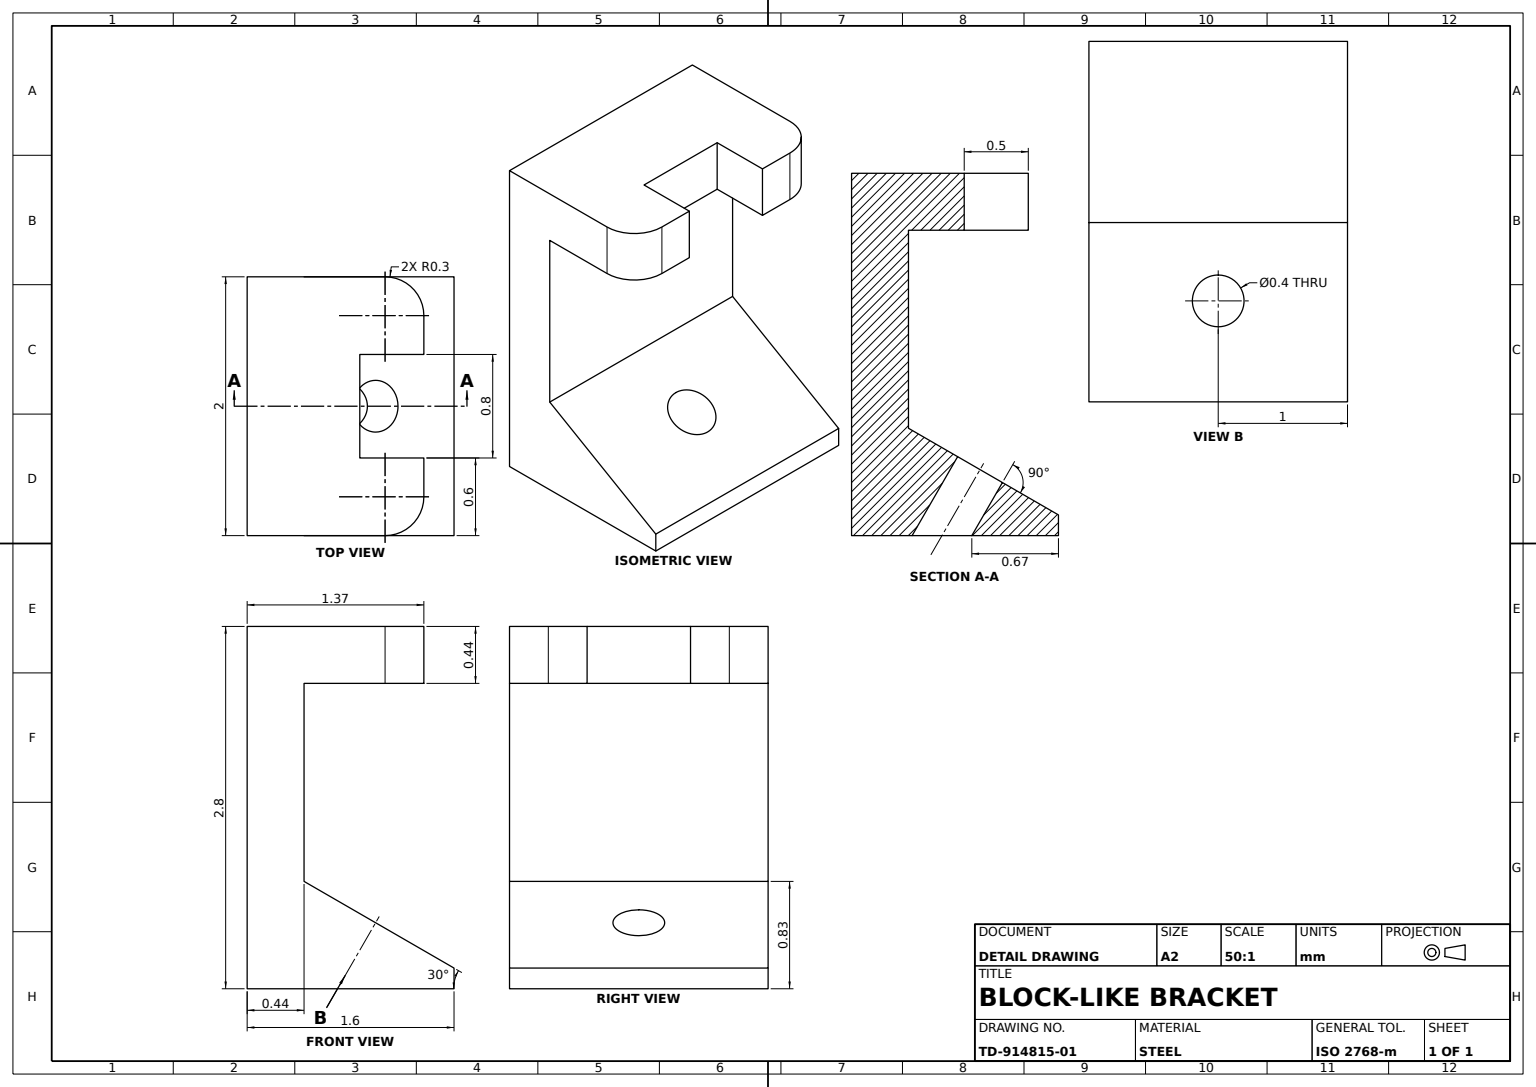
from build123d import *

# Parameters (mm, degrees)
BRACKET_BODY_DEPTH     = 1
CUT_0_4_SKETCH_R       = 0.2
CUT_0_4_THROUGH_DEPTH  = 2
NOTCH_0_8X0_5_SKETCH_W = 0.495523031
NOTCH_0_8X0_5_SKETCH_H = 0.799987473
NOTCH_0_8X0_5_DEPTH    = 0.5
PROFILED_NOTCH_DEPTH   = 0.5


with BuildPart() as part:
    # Bracket Profile Sketch → Bracket Body (new, symmetric)
    with BuildSketch(Plane.XY):
        Polygon((0, 0), (0, 1.4), (-1.36670697, 1.4), (-1.36670697, 0.96), (-0.44, 0.96), (-0.44, -0.570273688), (-1.6, -1.24), (-1.6, -1.4), (0, -1.4), align=None)
    extrude(amount=BRACKET_BODY_DEPTH, both=True)

    # Cut Ø0.4 Sketch → Cut Ø0.4 Through (cut)
    with BuildSketch(Plane(origin=(0.13693575, -0.237179677, 0), x_dir=(0.866025403784438, 0.5000000000000012, 0), z_dir=(-0.5000000000000012, 0.866025403784438, 0))):
        with Locations(Location((-1.30537787, 0, 0), (0, 0, 180))):
            Circle(CUT_0_4_SKETCH_R)
    extrude(amount=-CUT_0_4_THROUGH_DEPTH, mode=Mode.SUBTRACT)

    # Notch 0.8x0.5 Sketch → Notch 0.8x0.5 (cut)
    with BuildSketch(Plane(origin=(0, 1.4, 0), x_dir=(1, 0, 0), z_dir=(0, 1, 0))):
        with Locations((-1.118945454, 6.263e-06)):
            Rectangle(NOTCH_0_8X0_5_SKETCH_W, NOTCH_0_8X0_5_SKETCH_H)
    extrude(amount=-NOTCH_0_8X0_5_DEPTH, mode=Mode.SUBTRACT)

    # Profiled Notch Sketch → Profiled Notch (cut)
    with BuildSketch(Plane(origin=(0, 1.4, 0), x_dir=(1, 0, 0), z_dir=(0, 1, 0))):
        with BuildLine():
            Line((-1.36670697, 0.7), (-1.36670697, 1))
            Line((-1.36670697, 1), (-1.06670697, 1))
            ThreePointArc((-1.06670697, 1), (-1.278839005, 0.912132034), (-1.36670697, 0.7))
        make_face()
        with BuildLine():
            Line((-1.36670697, -0.7), (-1.36670697, -1))
            Line((-1.36670697, -1), (-1.06670697, -1))
            ThreePointArc((-1.06670697, -1), (-1.278839005, -0.912132034), (-1.36670697, -0.7))
        make_face()
    extrude(amount=-PROFILED_NOTCH_DEPTH, mode=Mode.SUBTRACT)


solid = part.part
